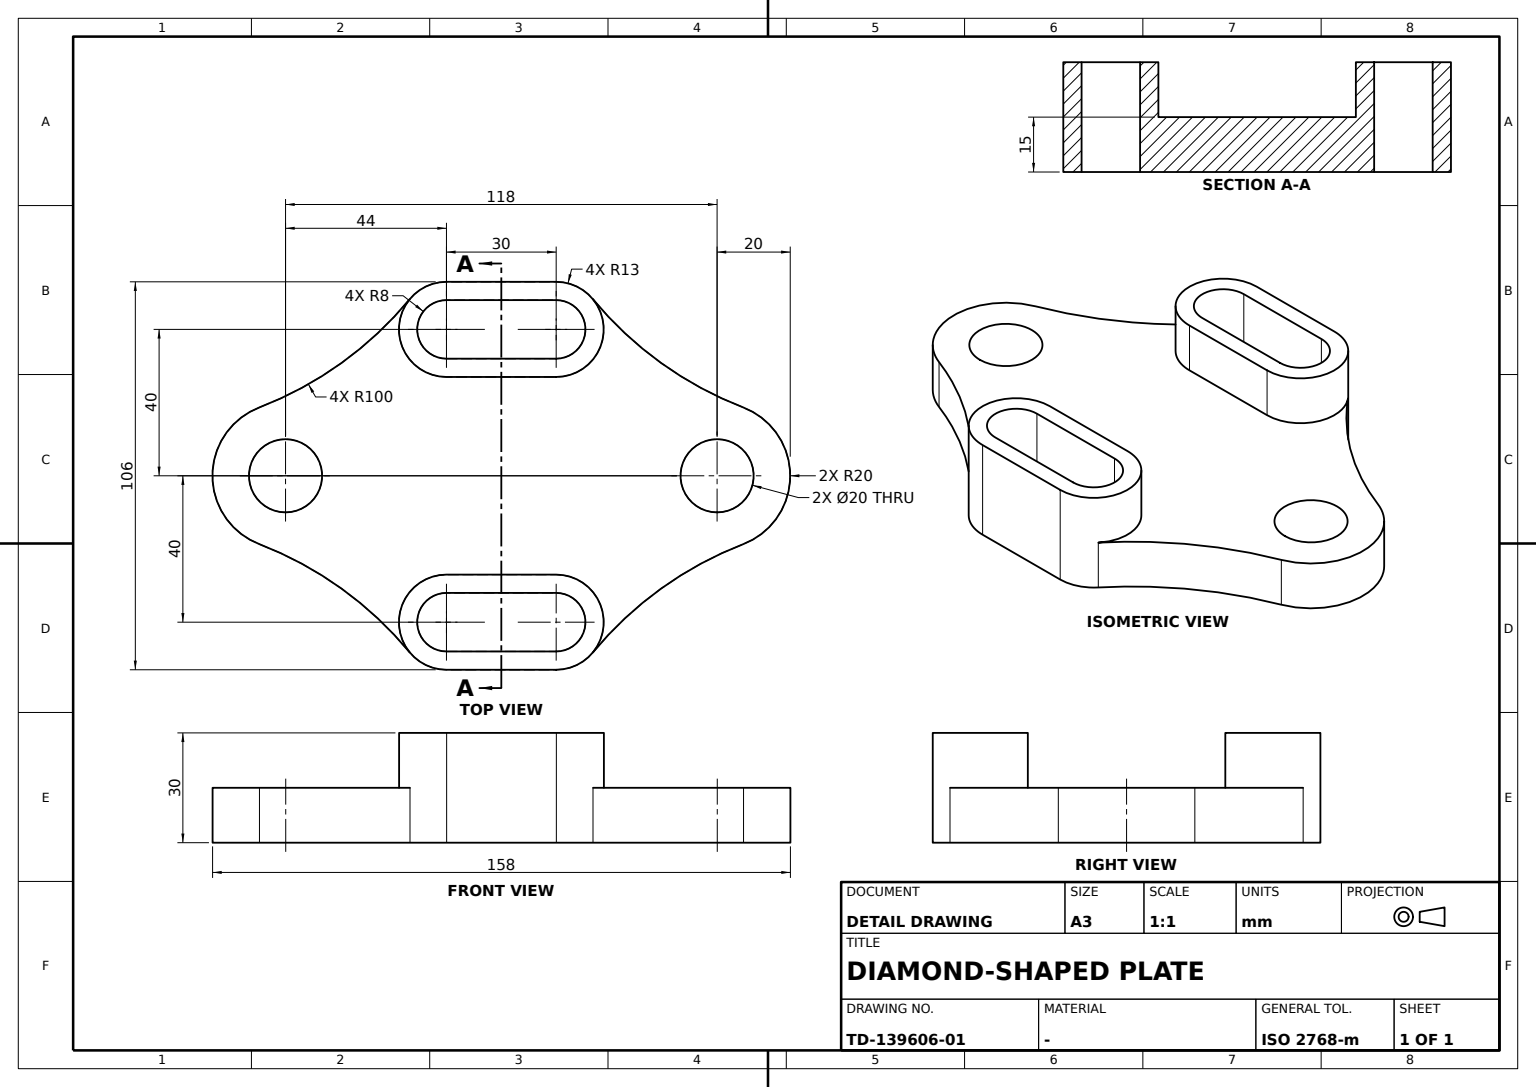
CATIA V5 part; units mm, degrees
sketch "Sketch1" plane through (0, 0, 0) normal (0, 0, 1) x (1, 0, 0)
  circle A0 centre (0, -59) radius 10
  point P0 (0, -59)
  circle A1 centre (0, 59) radius 10
  point P1 (0, 59)
  arc A2 (-18.6657, -66.1828) -> (18.6657, -66.1828) centre (0, -59) ccw
  arc A3 (18.6657, 66.1828) -> (-18.6657, 66.1828) centre (0, 59) ccw
  line L0 (40, 15) -> (40, -15) construction
  point P2 (40, -15)
  line L1 (53, 15) -> (53, -15)
  arc A4 (53, -15) -> (48.2825, -25.02) centre (40, -15) cw
  arc A5 (48.2825, 25.02) -> (53, 15) centre (40, 15) cw
  line L2 (-40, 15) -> (-40, -15) construction
  point P3 (-40, -15)
  line L3 (-53, -15) -> (-53, 15)
  arc A6 (-48.2825, -25.02) -> (-53, -15) centre (-40, -15) cw
  arc A7 (-53, 15) -> (-48.2825, 25.02) centre (-40, 15) cw
  arc A8 (18.6657, 66.1828) -> (48.2825, 25.02) centre (111.994, 102.0968) ccw
  arc A9 (48.2825, -25.02) -> (18.6657, -66.1828) centre (111.994, -102.0968) ccw
  arc A10 (-18.6657, -66.1828) -> (-48.2825, -25.02) centre (-111.994, -102.0968) ccw
  arc A11 (-48.2825, 25.02) -> (-18.6657, 66.1828) centre (-111.994, 102.0968) ccw
  dimension "radius A0" = 10
  dimension "radius A1" = 10
  dimension "radius A2" = 20
  dimension "radius A3" = 20
  dimension "distance P1 P0" = 118
  dimension "distance x axis P0" = 59
  dimension "radius A4" = 13
  dimension "distance L0 y axis" = 40
  dimension "length L0" = 30
  dimension "distance x axis P2" = 15
  dimension "radius A5" = 13
  dimension "length L2" = 30
  dimension "radius A6" = 13
  dimension "radius A7" = 13
  dimension "distance y axis L2" = 40
  dimension "distance P3 x axis" = 15
  dimension "radius A8" = 100
  dimension "radius A9" = 100
  dimension "radius A10" = 100
  dimension "radius A11" = 100
  constraint coincidence P0 y-axis
  constraint coincidence P1 y-axis
  constraint vertical L0 y-axis
  constraint vertical L2 y-axis
  constraint tangency A4 L1
  constraint tangency A5 L1
  constraint tangency A6 L3
  constraint tangency A7 L3
  constraint tangency A8 A3
  constraint tangency A8 A5
  constraint tangency A9 A4
  constraint tangency A9 A2
  constraint tangency A10 A6
  constraint tangency A10 A2
  constraint tangency A11 A3
  constraint tangency A11 A7
extrude "Pad1" add sketch "Sketch1" against normal blind 15
sketch "Sketch2" plane through (0, 0, 0) normal (0, 0, 1) x (1, 0, 0)
  arc A0 (48.2825, -25.02) -> (53, -15) centre (40, -15) ccw construction
  arc A1 (-53, -15) -> (-48.2825, -25.02) centre (-40, -15) ccw construction
  arc A2 (-48.2825, 25.02) -> (-53, 15) centre (-40, 15) ccw construction
  line L0 (40, 15) -> (40, -15) construction
  point P0 (40, -15)
  line L1 (53, 15) -> (53, -15)
  line L2 (27, -15) -> (27, 15)
  arc A3 (53, -15) -> (27, -15) centre (40, -15) cw
  arc A4 (27, 15) -> (53, 15) centre (40, 15) cw
  line L3 (-40, 15) -> (-40, -15) construction
  point P1 (-40, 15)
  point P2 (-40, -15)
  line L4 (-27, 15) -> (-27, -15)
  line L5 (-53, -15) -> (-53, 15)
  arc A5 (-27, -15) -> (-53, -15) centre (-40, -15) cw
  arc A6 (-53, 15) -> (-27, 15) centre (-40, 15) cw
  line L6 (40, 15) -> (40, -15) construction
  point P3 (40, -15)
  line L7 (48, 15) -> (48, -15)
  line L8 (32, -15) -> (32, 15)
  arc A7 (48, -15) -> (32, -15) centre (40, -15) cw
  arc A8 (32, 15) -> (48, 15) centre (40, 15) cw
  line L9 (-40, 15) -> (-40, -15) construction
  point P4 (-40, -15)
  line L10 (-32, 15) -> (-32, -15)
  line L11 (-48, -15) -> (-48, 15)
  arc A9 (-32, -15) -> (-48, -15) centre (-40, -15) cw
  arc A10 (-48, 15) -> (-32, 15) centre (-40, 15) cw
  dimension "length L0" = 30
  dimension "distance P0 x axis" = 15
  dimension "radius A4" = 13
  dimension "radius A3" = 13
  dimension "radius A6" = 13
  dimension "radius A5" = 13
  dimension "radius A8" = 8
  dimension "radius A7" = 8
  dimension "radius A10" = 8
  dimension "radius A9" = 8
  constraint vertical L0 y-axis
  constraint vertical L3 y-axis
  constraint vertical L6 y-axis
  constraint vertical L9 y-axis
  constraint tangency A3 L1
  constraint tangency A4 L1
  constraint tangency A3 L2
  constraint tangency A4 L2
  constraint tangency A5 L4
  constraint tangency A6 L4
  constraint tangency A5 L5
  constraint tangency A6 L5
  constraint tangency A7 L7
  constraint tangency A8 L7
  constraint tangency A7 L8
  constraint tangency A8 L8
  constraint tangency A9 L10
  constraint tangency A10 L10
  constraint tangency A9 L11
  constraint tangency A10 L11
  constraint concentricity P1 A2
  constraint concentricity P2 A1
  constraint concentricity P3 A0
  constraint concentricity P4 A1
extrude "Pad2" add sketch "Sketch2" along normal blind 15
sketch "Sketch3" plane through (0, 0, 0) normal (0, 0, 1) x (1, 0, 0)
  arc A0 (-48, -15) -> (-32, -15) centre (-40, -15) ccw
  line L0 (-48, 15) -> (-48, -15)
  arc A1 (-32, 15) -> (-48, 15) centre (-40, 15) ccw
  line L1 (-32, -15) -> (-32, 15)
  line L2 (32, 15) -> (32, -15)
  arc A2 (48, 15) -> (32, 15) centre (40, 15) ccw
  line L3 (48, -15) -> (48, 15)
  arc A3 (32, -15) -> (48, -15) centre (40, -15) ccw
extrude "Pocket1" cut sketch "Sketch3" against normal blind 15
